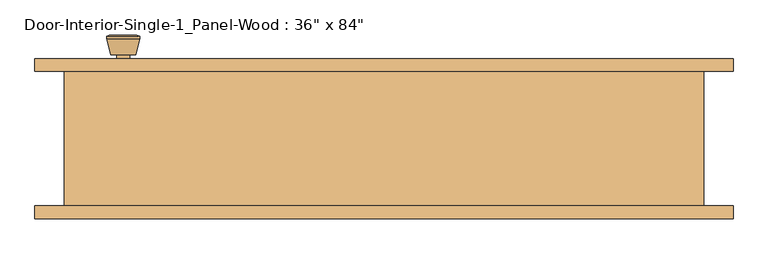
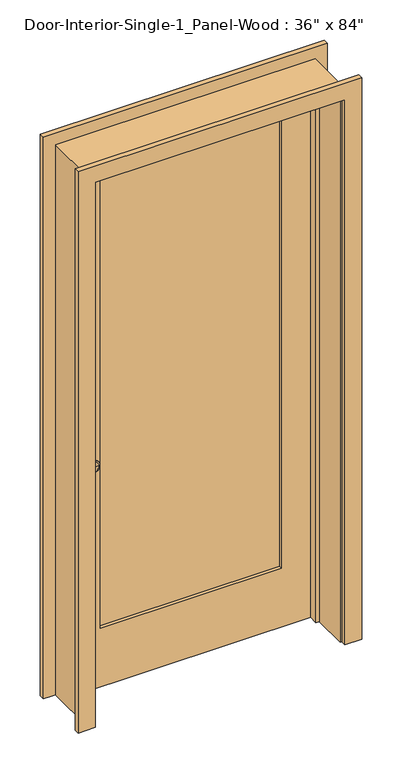
"""IFC4 building model written with IfcOpenShell, lengths in millimetres: door geometry."""

from ifc_helpers import new_model, si_unit, point, frame, frame_2d, origin, place, context, project, spatial, polyline, circle_curve, trimmed, segment, composite_curve, outline, extrude, faceted_brep, source, transform, mapped, element, save
from ifc_brep_helpers import plane_surface, cylinder_surface, revolved_surface, advanced_brep


def door_9c4ddfbd(model_context):
    return source(origin(), model_context, "Body", "SolidModel", [
        advanced_brep(
        [(-393.7, 57.5, 914.4), (-383.7, 57.5, 914.4), (-403.7, 57.5, 914.4), (-373.2241324, 8.5, 914.4), (-393.7, 8.5, 914.4), (-414.1758676, 8.5, 914.4), (-368.7, 10.3278681, 914.4), (-418.7, 10.3278681, 914.4), (-368.7, 13.7915463, 914.4), (-418.7, 13.7915463, 914.4), (-375.063764, 38.5, 914.4), (-412.336236, 38.5, 914.4), (-383.7, 38.5, 914.4), (-403.7, 38.5, 914.4)],
        [
            (0, 1),
            (1, 2, circle_curve(frame((-393.7, 57.5, 914.4), z_axis=(0.0, 1.0, 0.0), x_axis=(-1.0, 0.0, 0.0)), 10.0)),
            (2, 0),
            (2, 1, circle_curve(frame((-393.7, 57.5, 914.4), z_axis=(0.0, 1.0, 0.0), x_axis=(-1.0, 0.0, 0.0)), 10.0)),
            (3, 4),
            (4, 5),
            (5, 3, circle_curve(frame((-393.7, 8.5, 914.4), z_axis=(0.0, -1.0, 0.0), x_axis=(-1.0, 0.0, 0.0)), 20.4758676)),
            (3, 5, circle_curve(frame((-393.7, 8.5, 914.4), z_axis=(0.0, -1.0, 0.0), x_axis=(-1.0, 0.0, 0.0)), 20.4758676)),
            (6, 3),
            (5, 7),
            (7, 6, circle_curve(frame((-393.7, 10.3278681, 914.4), z_axis=(0.0, -1.0, 0.0), x_axis=(-1.0, 0.0, 0.0)), 25.0)),
            (6, 7, circle_curve(frame((-393.7, 10.3278681, 914.4), z_axis=(0.0, -1.0, 0.0), x_axis=(-1.0, 0.0, 0.0)), 25.0)),
            (8, 6),
            (7, 9),
            (9, 8, circle_curve(frame((-393.7, 13.7915463, 914.4), z_axis=(0.0, -1.0, 0.0), x_axis=(-1.0, 0.0, 0.0)), 25.0)),
            (8, 9, circle_curve(frame((-393.7, 13.7915463, 914.4), z_axis=(0.0, -1.0, 0.0), x_axis=(-1.0, 0.0, 0.0)), 25.0)),
            (10, 8),
            (9, 11),
            (11, 10, circle_curve(frame((-393.7, 38.5, 914.4), z_axis=(0.0, -1.0, 0.0), x_axis=(-1.0, 0.0, 0.0)), 18.636236)),
            (10, 11, circle_curve(frame((-393.7, 38.5, 914.4), z_axis=(0.0, -1.0, 0.0), x_axis=(-1.0, 0.0, 0.0)), 18.636236)),
            (12, 10),
            (11, 13),
            (13, 12, circle_curve(frame((-393.7, 38.5, 914.4), z_axis=(0.0, -1.0, 0.0), x_axis=(-1.0, 0.0, 0.0)), 10.0)),
            (12, 13, circle_curve(frame((-393.7, 38.5, 914.4), z_axis=(0.0, -1.0, 0.0), x_axis=(-1.0, 0.0, 0.0)), 10.0)),
            (1, 12),
            (13, 2),
        ],
        [
            plane_surface(frame((-393.7, 57.5, 914.4), z_axis=(0.0, 1.0, 0.0), x_axis=(-1.0, 0.0, 0.0))),
            plane_surface(frame((-393.7, 8.5, 914.4), z_axis=(0.0, -1.0, 0.0), x_axis=(-1.0, 0.0, 0.0))),
            revolved_surface(polyline([(-414.1758676, 8.5, 914.4), (-418.7, 10.3278681, 914.4)]), (-393.7, 57.5, 914.4), (0.0, 1.0, 0.0)),
            cylinder_surface(frame((-393.7, 57.5, 914.4), z_axis=(0.0, 1.0, 0.0), x_axis=(-1.0, 0.0, 0.0)), 25.0),
            revolved_surface(polyline([(-418.7, 13.7915463, 914.4), (-412.336236, 38.5, 914.4)]), (-393.7, 57.5, 914.4), (0.0, 1.0, 0.0)),
            plane_surface(frame((-393.7, 38.5, 914.4), z_axis=(0.0, 1.0, 0.0), x_axis=(-1.0, 0.0, 0.0))),
            cylinder_surface(frame((-393.7, 57.5, 914.4), z_axis=(0.0, 1.0, 0.0), x_axis=(-1.0, 0.0, 0.0)), 10.0),
        ],
        [
            (0, [[1, 2, 3]]),
            (0, [[-3, 4, -1]]),
            (1, [[5, 6, 7]]),
            (1, [[-6, -5, 8]]),
            (2, [[9, -7, 10, 11]]),
            (2, [[-10, -8, -9, 12]]),
            (3, [[13, -11, 14, 15]]),
            (3, [[-14, -12, -13, 16]]),
            (4, [[17, -15, 18, 19]]),
            (4, [[-18, -16, -17, 20]]),
            (5, [[21, -19, 22, 23]]),
            (5, [[-22, -20, -21, 24]]),
            (6, [[25, -23, 26, -2]]),
            (6, [[-26, -24, -25, -4]]),
        ],
    ),
        extrude(outline(composite_curve([segment(trimmed(circle_curve(frame_2d((914.4, -393.7)), 30.0), [point((914.4, -423.7))], [point((914.4, -363.7))], False, "CARTESIAN"), True, "CONTINUOUS"), segment(trimmed(circle_curve(frame_2d((914.4, -393.7)), 30.0), [point((914.4, -363.7))], [point((914.4, -423.7))], False, "CARTESIAN"), True, "CONTINUOUS")], self_intersect=False)), frame((0.0, 57.5, 0.0), z_axis=(0.0, 1.0, 0.0), x_axis=(0.0, 0.0, 1.0)), (0.0, 0.0, 1.0), 6.0),
        advanced_brep(
        [(-393.7, 104.425, 914.4), (-403.7, 104.425, 914.4), (-383.7, 104.425, 914.4), (-373.2241324, 153.425, 914.4), (-414.1758676, 153.425, 914.4), (-393.7, 153.425, 914.4), (-368.7, 151.5971319, 914.4), (-418.7, 151.5971319, 914.4), (-368.7, 148.1334537, 914.4), (-418.7, 148.1334537, 914.4), (-375.063764, 123.425, 914.4), (-412.336236, 123.425, 914.4), (-383.7, 123.425, 914.4), (-403.7, 123.425, 914.4)],
        [
            (0, 1),
            (1, 2, circle_curve(frame((-393.7, 104.425, 914.4), z_axis=(0.0, -1.0, 0.0), x_axis=(-1.0, 0.0, 0.0)), 10.0)),
            (2, 0),
            (2, 1, circle_curve(frame((-393.7, 104.425, 914.4), z_axis=(0.0, -1.0, 0.0), x_axis=(-1.0, 0.0, 0.0)), 10.0)),
            (3, 4, circle_curve(frame((-393.7, 153.425, 914.4), z_axis=(0.0, 1.0, 0.0), x_axis=(-1.0, 0.0, 0.0)), 20.4758676)),
            (4, 5),
            (5, 3),
            (4, 3, circle_curve(frame((-393.7, 153.425, 914.4), z_axis=(0.0, 1.0, 0.0), x_axis=(-1.0, 0.0, 0.0)), 20.4758676)),
            (6, 7, circle_curve(frame((-393.7, 151.5971319, 914.4), z_axis=(0.0, 1.0, 0.0), x_axis=(-1.0, 0.0, 0.0)), 25.0)),
            (7, 4),
            (3, 6),
            (7, 6, circle_curve(frame((-393.7, 151.5971319, 914.4), z_axis=(0.0, 1.0, 0.0), x_axis=(-1.0, 0.0, 0.0)), 25.0)),
            (8, 9, circle_curve(frame((-393.7, 148.1334537, 914.4), z_axis=(0.0, 1.0, 0.0), x_axis=(-1.0, 0.0, 0.0)), 25.0)),
            (9, 7),
            (6, 8),
            (9, 8, circle_curve(frame((-393.7, 148.1334537, 914.4), z_axis=(0.0, 1.0, 0.0), x_axis=(-1.0, 0.0, 0.0)), 25.0)),
            (10, 11, circle_curve(frame((-393.7, 123.425, 914.4), z_axis=(0.0, 1.0, 0.0), x_axis=(-1.0, 0.0, 0.0)), 18.636236)),
            (11, 9),
            (8, 10),
            (11, 10, circle_curve(frame((-393.7, 123.425, 914.4), z_axis=(0.0, 1.0, 0.0), x_axis=(-1.0, 0.0, 0.0)), 18.636236)),
            (12, 13, circle_curve(frame((-393.7, 123.425, 914.4), z_axis=(0.0, 1.0, 0.0), x_axis=(-1.0, 0.0, 0.0)), 10.0)),
            (13, 11),
            (10, 12),
            (13, 12, circle_curve(frame((-393.7, 123.425, 914.4), z_axis=(0.0, 1.0, 0.0), x_axis=(-1.0, 0.0, 0.0)), 10.0)),
            (1, 13),
            (12, 2),
        ],
        [
            plane_surface(frame((-393.7, 104.425, 914.4), z_axis=(0.0, -1.0, 0.0), x_axis=(-1.0, 0.0, 0.0))),
            plane_surface(frame((-393.7, 153.425, 914.4), z_axis=(0.0, 1.0, 0.0), x_axis=(-1.0, 0.0, 0.0))),
            revolved_surface(polyline([(-414.1758676, 153.425, 914.4), (-418.7, 151.5971319, 914.4)]), (-393.7, 104.425, 914.4), (0.0, -1.0, 0.0)),
            cylinder_surface(frame((-393.7, 104.425, 914.4), z_axis=(0.0, -1.0, 0.0), x_axis=(-1.0, 0.0, 0.0)), 25.0),
            revolved_surface(polyline([(-418.7, 148.1334537, 914.4), (-412.336236, 123.425, 914.4)]), (-393.7, 104.425, 914.4), (0.0, -1.0, 0.0)),
            plane_surface(frame((-393.7, 123.425, 914.4), z_axis=(0.0, -1.0, 0.0), x_axis=(-1.0, 0.0, 0.0))),
            cylinder_surface(frame((-393.7, 104.425, 914.4), z_axis=(0.0, -1.0, 0.0), x_axis=(-1.0, 0.0, 0.0)), 10.0),
        ],
        [
            (0, [[1, 2, 3]]),
            (0, [[-3, 4, -1]]),
            (1, [[5, 6, 7]]),
            (1, [[8, -7, -6]]),
            (2, [[9, 10, -5, 11]]),
            (2, [[12, -11, -8, -10]]),
            (3, [[13, 14, -9, 15]]),
            (3, [[16, -15, -12, -14]]),
            (4, [[17, 18, -13, 19]]),
            (4, [[20, -19, -16, -18]]),
            (5, [[21, 22, -17, 23]]),
            (5, [[24, -23, -20, -22]]),
            (6, [[-2, 25, -21, 26]]),
            (6, [[-4, -26, -24, -25]]),
        ],
    ),
        extrude(outline(composite_curve([segment(trimmed(circle_curve(frame_2d((914.4, -393.7)), 30.0), [point((914.4, -423.7))], [point((914.4, -363.7))], False, "CARTESIAN"), True, "CONTINUOUS"), segment(trimmed(circle_curve(frame_2d((914.4, -393.7)), 30.0), [point((914.4, -363.7))], [point((914.4, -423.7))], False, "CARTESIAN"), True, "CONTINUOUS")], self_intersect=False)), frame((0.0, 98.425, 0.0), z_axis=(0.0, 1.0, 0.0), x_axis=(0.0, 0.0, 1.0)), (0.0, 0.0, 1.0), 6.0),
        faceted_brep([(482.6, 98.425, 0.0), (482.6, -104.775, 0.0), (457.2, -104.775, 0.0), (457.2, 28.575, 0.0), (444.5, 28.575, 0.0), (444.5, 63.5, 0.0), (457.2, 63.5, 0.0), (457.2, 98.425, 0.0), (482.6, 98.425, 2159.0), (482.6, -104.775, 2159.0), (-482.6, -104.775, 2159.0), (-482.6, -104.775, 0.0), (-457.2, -104.775, 0.0), (-457.2, -104.775, 2133.6), (457.2, -104.775, 2133.6), (457.2, 28.575, 2133.6), (-457.2, 28.575, 2133.6), (-457.2, 28.575, 0.0), (-444.5, 28.575, 0.0), (-444.5, 28.575, 2120.9), (444.5, 28.575, 2120.9), (444.5, 63.5, 2120.9), (-444.5, 63.5, 2120.9), (-444.5, 63.5, 0.0), (-457.2, 63.5, 0.0), (-457.2, 63.5, 2133.6), (457.2, 63.5, 2133.6), (457.2, 98.425, 2133.6), (-457.2, 98.425, 2133.6), (-457.2, 98.425, 0.0), (-482.6, 98.425, 0.0), (-482.6, 98.425, 2159.0)], [[[0, 1, 2, 3, 4, 5, 6, 7]], [[1, 0, 8, 9]], [[2, 1, 9, 10, 11, 12, 13, 14]], [[3, 2, 14, 15]], [[4, 3, 15, 16, 17, 18, 19, 20]], [[5, 4, 20, 21]], [[6, 5, 21, 22, 23, 24, 25, 26]], [[7, 6, 26, 27]], [[0, 7, 27, 28, 29, 30, 31, 8]], [[9, 8, 31, 10]], [[15, 14, 13, 16]], [[21, 20, 19, 22]], [[27, 26, 25, 28]], [[30, 29, 24, 23, 18, 17, 12, 11]], [[10, 31, 30, 11]], [[16, 13, 12, 17]], [[22, 19, 18, 23]], [[28, 25, 24, 29]]]),
        extrude(outline(polyline([(2133.6, -457.2), (0.0, -457.2), (0.0, 457.2), (2133.6, 457.2), (2133.6, -457.2)]), holes=[polyline([(2014.5375, -336.55), (2014.5375, 336.55), (231.775, 336.55), (231.775, -336.55), (2014.5375, -336.55)])]), frame((0.0, 63.5, 0.0), z_axis=(0.0, 1.0, 0.0), x_axis=(0.0, 0.0, 1.0)), (0.0, 0.0, 1.0), 34.925),
        extrude(outline(polyline([(336.55, 75.1416667), (-336.55, 75.1416667), (-336.55, 86.7833333), (336.55, 86.7833333), (336.55, 75.1416667)])), frame((0.0, 0.0, 231.775), z_axis=(0.0, 0.0, 1.0), x_axis=(1.0, 0.0, 0.0)), (0.0, 0.0, 1.0), 1782.7625),
        extrude(outline(polyline([(0.0, 463.55), (0.0, 527.05), (2203.45, 527.05), (2203.45, -527.05), (0.0, -527.05), (0.0, -463.55), (2139.95, -463.55), (2139.95, 463.55), (0.0, 463.55)])), frame((0.0, 98.425, 0.0), z_axis=(0.0, 1.0, 0.0), x_axis=(0.0, 0.0, 1.0)), (0.0, 0.0, 1.0), 19.05),
        extrude(outline(polyline([(0.0, 463.55), (0.0, 527.05), (2203.45, 527.05), (2203.45, -527.05), (0.0, -527.05), (0.0, -463.55), (2139.95, -463.55), (2139.95, 463.55), (0.0, 463.55)])), frame((0.0, -123.825, 0.0), z_axis=(0.0, 1.0, 0.0), x_axis=(0.0, 0.0, 1.0)), (0.0, 0.0, 1.0), 19.05),
    ])


if __name__ == "__main__":
    model = new_model("IFC4")
    model_context = context("Model", 3, world=origin())
    ifc_project = project(units=[si_unit("LENGTHUNIT", "METRE", prefix="MILLI")], contexts=[model_context])
    site = spatial("IfcSite", under=ifc_project)
    building = spatial("IfcBuilding", under=site)
    placement = place(None, origin())
    door_shape = door_9c4ddfbd(model_context)
    element("IfcDoor", 1, ObjectType="Door-Interior-Single-1_Panel-Wood : 36\" x 84\"", at=placement, inside=building, context=model_context, shape_type="MappedRepresentation", body=[
        mapped(door_shape, transform((0.0, 0.0, 0.0), x_axis=(1.0, 0.0, 0.0), y_axis=(0.0, 1.0, 0.0), z_axis=(0.0, 0.0, 1.0))),
    ])
    save(model, "model.ifc")

# Revit data of these elements
# Type "Door-Interior-Single-1_Panel-Wood : 36\" x 84\""
#   Type Mark = "10"
#   Analytic Construction = "Wooden"
#   Top Rail = 0' - 4 11/16"
#   Thickness = 0' - 1 3/8"
#   Thermal Resistance (R) = 2.5876 (h·ft²·°F)/BTU
#   Swing Angle [instance default] = 90.00°
#   Stiles = 0' - 4 3/4"
#   Rough Width = 3' - 2"
#   Rough Height = 7' - 1"
#   Height = 7' - 0"
#   Width = 3' - 0"
#   Heat Transfer Coefficient (U) = 0.3865 BTU/(h·ft²·°F)
#   Bottom Rail = 0' - 9 1/8"
#   Trim Material = Cherry
#   Panel Material = Cherry
#   Frame Material = Cherry
#   Door Handle Material = Aluminum
#   Visual Light Transmittance = 0
#   Solar Heat Gain Coefficient = 0
#   Wall Closure = (empty or 0)
#   Function = (empty or 0)
# Element 1 (IfcDoor, "Door-Interior-Single-1_Panel-Wood : 36\" x 84\"")
#   Materials on its faces: "Cherry", "Aluminum"
# Materials
#   "Cherry": class "Wood", colour RGB 226 177 128, transparency 0, Description = "Prunus Serotina", Cost = 0
#   "Aluminum": class "Metal", colour RGB 247 247 247, transparency 0, Description = "Aluminum 6061", Cost = 0
